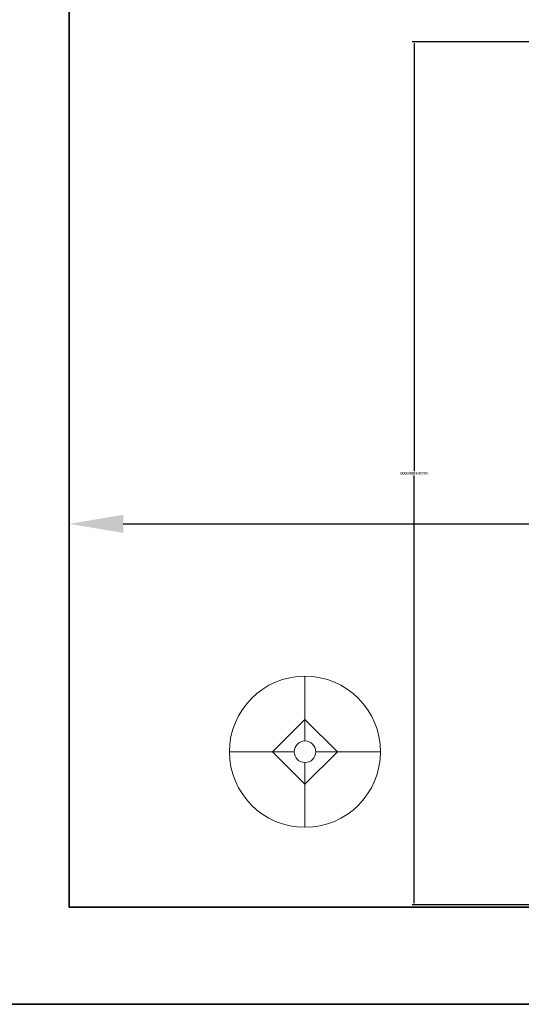
# Model space of a CAD drawing. Units: inches. Extents: x -128 to 854, y -395 to 398.
# Tile 23 of 61: x 152 to 199, y -89 to 2. Entities that reach past the tile are written whole.
import ezdxf

# ---------------------------------------------------------------- set-up
doc = ezdxf.new("R2010")
doc.units = ezdxf.units.IN
doc.header["$MEASUREMENT"] = 0
for name, color, linetype, lineweight in [('A-ANNO-DIMS', 2, 'Continuous', 18), ('A-FURN', 8, 'Continuous', 18), ('A-WALL', 4, 'Continuous', 35)]:
    doc.layers.add(name, color=color, linetype=linetype, lineweight=lineweight)
doc.styles.get("Standard").update_dxf_attribs({"font": 'arial.ttf'})
doc.dimstyles.get("Standard").update_dxf_attribs({"dimtxt": 0.18, "dimasz": 0.18, "dimexe": 0.18, "dimexo": 0.0625, "dimgap": 0.09, "dimtad": 0, "dimtih": 1, "dimtoh": 1, "dimdec": 1, "dimzin": 0, "dimdsep": 46, "dimlunit": 4, "dimtxsty": 'Standard', "dimcen": 0.09, "dimclrd": 1, "dimclre": 2, "dimclrt": 6, "dimadec": 0, "dimazin": 0, "dimtfac": 1, "dimtdec": 1, "dimtofl": 0, "dimtmove": 0, "dimatfit": 3, "dimfxl": 1, "dimtfill": 2, "dimtfillclr": 3, "dimtolj": 1, "dimtzin": 0, "dimarcsym": 0})

# ---------------------------------------------------------------- blocks, each defined once
blk = doc.blocks.new('Lamp - Table')
for p, q in [((0, 7), (0, 1)), ((0, 3), (-3, 0)), ((3, 0), (0, 3)), ((-1, 0), (-7, 0)), ((-3, 0), (0, -3)), ((0, -3), (3, 0)), ((1, 0), (7, 0)), ((0, -1), (0, -7))]:
    blk.add_line(p, q)
for radius in [7, 1]:
    blk.add_circle((0, 0), radius)
blk = doc.blocks.new('*D43')
at = {"layer": 'A-ANNO-DIMS', "color": 0, "lineweight": -2, "transparency": 16777216}
for p, q in [((156.873, -80.197), (156.873, -44.559)), ((304.873, -80.197), (304.873, -44.559)), ((161.873, -44.739), (224.101, -44.739)), ((299.873, -44.739), (237.645, -44.739))]:
    blk.add_line(p, q, dxfattribs=at)
at = {"layer": 'A-ANNO-DIMS', "color": 0, "transparency": 16777216}
for points in [[(161.873, -43.906), (161.873, -45.572), (156.873, -44.739)], [(299.873, -43.906), (299.873, -45.572), (304.873, -44.739)]]:
    blk.add_solid(points, dxfattribs=at)
at = {"layer": 'Defpoints', "color": 0, "transparency": 16777216}
for p in [(304.873, -44.739), (156.873, -80.259), (304.873, -80.259)]:
    blk.add_point(p, dxfattribs=at)
at = {"layer": 'A-ANNO-DIMS', "color": 0, "transparency": 16777216, "insert": (230.873, -44.739), "char_height": 4, "attachment_point": 5, "bg_fill": 1, "box_fill_scale": 1.25, "bg_fill_color": 3, "bg_fill_transparency": 0}
blk.add_mtext('\\A1;12\'-4"', dxfattribs=at)
blk = doc.blocks.new('*D77')
at = {"layer": 'A-ANNO-DIMS', "color": 2, "lineweight": -2, "transparency": 16777216}
for p, q in [((200.764, -0.056), (188.647, -0.056)), ((200.764, -80.056), (188.647, -80.056))]:
    blk.add_line(p, q, dxfattribs=at)
at = {"layer": 'A-ANNO-DIMS', "color": 1, "lineweight": -2, "transparency": 16777216}
for p, q in [((188.827, -0.236), (188.827, -39.867)), ((188.827, -79.876), (188.827, -40.245))]:
    blk.add_line(p, q, dxfattribs=at)
at = {"layer": 'A-ANNO-DIMS', "color": 1, "transparency": 16777216}
for points in [[(188.797, -0.236), (188.857, -0.236), (188.827, -0.056)], [(188.797, -79.876), (188.857, -79.876), (188.827, -80.056)]]:
    blk.add_solid(points, dxfattribs=at)
at = {"layer": 'Defpoints', "color": 0, "transparency": 16777216}
for p in [(200.827, -0.056), (188.827, -80.056), (200.827, -80.056)]:
    blk.add_point(p, dxfattribs=at)
at = {"layer": 'A-ANNO-DIMS', "color": 6, "transparency": 16777216, "insert": (188.827, -40.056), "char_height": 0.18, "attachment_point": 5, "bg_fill": 1, "box_fill_scale": 1.25, "bg_fill_color": 3, "bg_fill_transparency": 0}
blk.add_mtext('\\A1;QUEEN BED 6\'-8" TYP.', dxfattribs=at)

msp = doc.modelspace()

# ---------------------------------------------------------------- linework, layer by layer
at = {"layer": 'A-WALL'}
for p, q in [((156.873, 72.741), (156.873, -80.259)), ((156.873, -80.259), (304.873, -80.259)), ((82.9, -89.259), (156.873, -89.259)), ((156.873, -89.259), (313.873, -89.259))]:
    msp.add_line(p, q, dxfattribs=at)

# ---------------------------------------------------------------- block references
at = {"layer": 'A-FURN'}
msp.add_blockref('Lamp - Table', (178.714, -65.856), dxfattribs=at)

# ---------------------------------------------------------------- dimensions: what is measured, and where the dimension line sits
at = {"layer": 'A-ANNO-DIMS'}
dim = msp.add_linear_dim(base=(188.827, -80.056), p1=(200.827, -0.056), p2=(200.827, -80.056), angle=270, text='QUEEN BED <> TYP.', dimstyle='Standard', override={"dimdec": 1, "dimlfac": 1, "dimrnd": 0, "dimzin": 1, "dimdsep": 46, "dimlunit": 4, "dimfrac": 2}, dxfattribs=at)
dim.commit()
dim.dimension.update_dxf_attribs({"geometry": '*D77', "text_midpoint": (188.827, -40.056)})
dim = msp.add_linear_dim(base=(304.873, -44.739), p1=(156.873, -80.259), p2=(304.873, -80.259), dimstyle='Standard', override={"dimtxt": 4, "dimasz": 5, "dimclrd": 0, "dimclre": 0, "dimclrt": 0}, dxfattribs=at)
dim.commit()
dim.dimension.update_dxf_attribs({"geometry": '*D43', "text_midpoint": (230.873, -44.739)})

doc.saveas('drawing.dxf')
